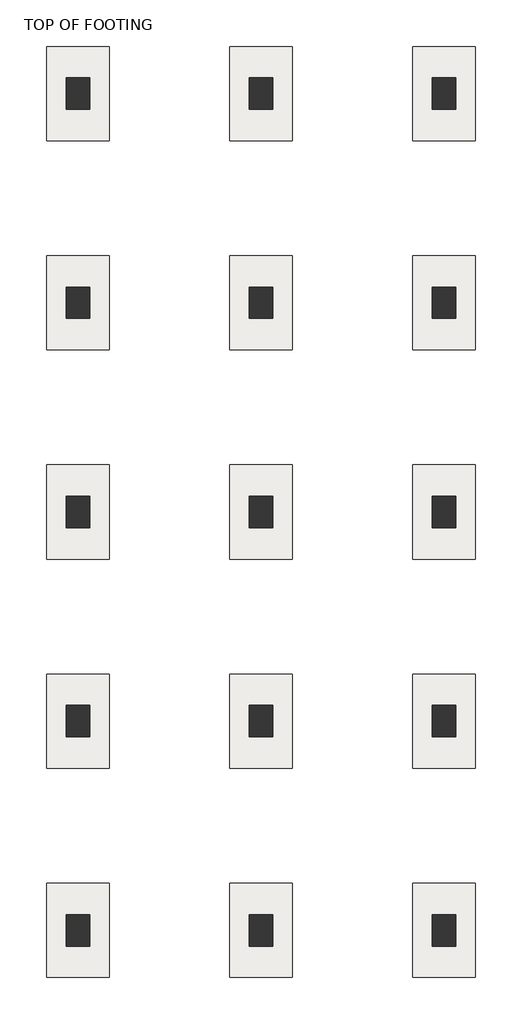
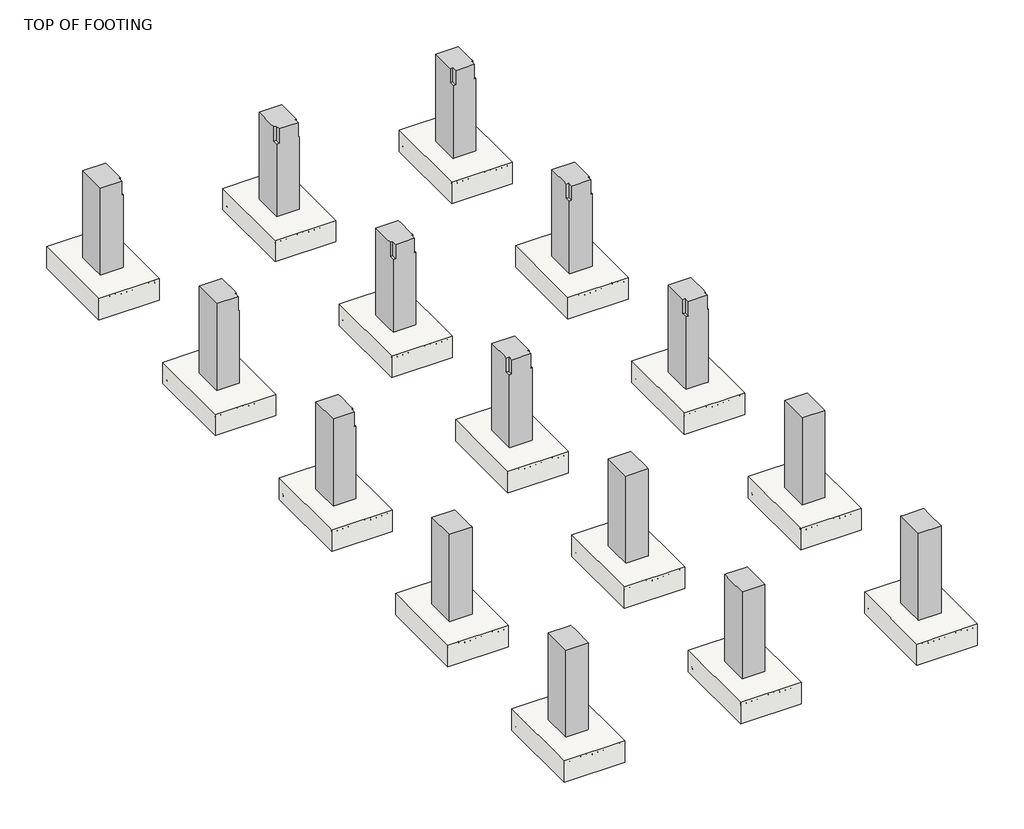
# One storey, part 1 of 11: 15 columns, 15 slabs.
"""IFC4 building model written with IfcOpenShell, lengths in millimetres."""

from ifc_helpers import new_model, si_unit, origin, place, context, project, spatial, faceted_brep, transform, mapped, element, save
from components import m_footing_rectangular_1800_x_1200_x_450mm_16ba7ea5

model = new_model("IFC4")

# Units and contexts
model_context = context("Model", 3, world=origin())
ifc_project = project(units=[si_unit("LENGTHUNIT", "METRE", prefix="MILLI")], contexts=[model_context])

# Site, building, storey
site = spatial("IfcSite", under=ifc_project)
building = spatial("IfcBuilding", under=site)
storey = spatial("IfcBuildingStorey", under=building, Name="TOP OF FOOTING", Elevation=-1828.8)

# Columns
placement = place(None, origin())
element("IfcColumn", 1, ObjectType="M_Concrete-Rectangular-Column : 450 x 600mm", at=placement, inside=storey, context=model_context, shape_type="Brep", body=[
    faceted_brep([(-9144.8884094, 19703.1212443, -1828.8), (-9144.8884094, 19103.1212443, -1828.8), (-9594.8884094, 19103.1212443, -1828.8), (-9594.8884094, 19703.1212443, -1828.8), (-9144.8884094, 19703.1212443, 0.0), (-9144.8884094, 19303.1212443, 0.0), (-9144.8884094, 19203.1212443, 0.0), (-9144.8884094, 19203.1212443, -300.0), (-9144.8884094, 19103.1212443, -300.0), (-9169.8884094, 19103.1212443, -300.0), (-9169.8884094, 19103.1212443, 0.0), (-9594.8884094, 19103.1212443, 0.0), (-9594.8884094, 19703.1212443, 0.0), (-9169.8884094, 19203.1212443, 0.0), (-9169.8884094, 19203.1212443, -300.0)], [[[0, 1, 2, 3]], [[1, 0, 4, 5, 6, 7, 8]], [[2, 1, 8, 9, 10, 11]], [[3, 2, 11, 12]], [[0, 3, 12, 4]], [[12, 11, 10, 13, 6, 5, 4]], [[7, 14, 9, 8]], [[14, 13, 10, 9]], [[14, 7, 6, 13]]]),
])
element("IfcColumn", 2, ObjectType="M_Concrete-Rectangular-Column : 450 x 600mm", at=placement, inside=storey, context=model_context, shape_type="Brep", body=[
    faceted_brep([(-5644.8884094, 19703.1212443, -1828.8), (-5644.8884094, 19103.1212443, -1828.8), (-6094.8884094, 19103.1212443, -1828.8), (-6094.8884094, 19703.1212443, -1828.8), (-5644.8884094, 19703.1212443, 0.0), (-5644.8884094, 19303.1212443, 0.0), (-5644.8884094, 19203.1212443, 0.0), (-5644.8884094, 19203.1212443, -300.0), (-5644.8884094, 19103.1212443, -300.0), (-5669.8884094, 19103.1212443, -300.0), (-5669.8884094, 19103.1212443, 0.0), (-6044.8884094, 19103.1212443, 0.0), (-6044.8884094, 19103.1212443, -300.0), (-6094.8884094, 19103.1212443, -300.0), (-6094.8884094, 19203.1212443, -300.0), (-6094.8884094, 19203.1212443, 0.0), (-6094.8884094, 19303.1212443, 0.0), (-6094.8884094, 19703.1212443, 0.0), (-6044.8884094, 19203.1212443, 0.0), (-5669.8884094, 19203.1212443, 0.0), (-5669.8884094, 19203.1212443, -300.0), (-6044.8884094, 19203.1212443, -300.0)], [[[0, 1, 2, 3]], [[1, 0, 4, 5, 6, 7, 8]], [[2, 1, 8, 9, 10, 11, 12, 13]], [[3, 2, 13, 14, 15, 16, 17]], [[0, 3, 17, 4]], [[4, 17, 16, 15, 18, 11, 10, 19, 6, 5]], [[7, 20, 9, 8]], [[20, 19, 10, 9]], [[20, 7, 6, 19]], [[21, 14, 13, 12]], [[18, 21, 12, 11]], [[14, 21, 18, 15]]]),
])
element("IfcColumn", 3, ObjectType="M_Concrete-Rectangular-Column : 450 x 600mm", at=placement, inside=storey, context=model_context, shape_type="Brep", body=[
    faceted_brep([(-2144.8884094, 19703.1212443, -1828.8), (-2144.8884094, 19103.1212443, -1828.8), (-2594.8884094, 19103.1212443, -1828.8), (-2594.8884094, 19703.1212443, -1828.8), (-2144.8884094, 19703.1212443, 0.0), (-2144.8884094, 19303.1212443, 0.0), (-2144.8884094, 19203.1212443, 0.0), (-2144.8884094, 19203.1212443, -300.0), (-2144.8884094, 19103.1212443, -300.0), (-2169.8884094, 19103.1212443, -300.0), (-2169.8884094, 19103.1212443, 0.0), (-2544.8884094, 19103.1212443, 0.0), (-2544.8884094, 19103.1212443, -300.0), (-2594.8884094, 19103.1212443, -300.0), (-2594.8884094, 19203.1212443, -300.0), (-2594.8884094, 19203.1212443, 0.0), (-2594.8884094, 19303.1212443, 0.0), (-2594.8884094, 19703.1212443, 0.0), (-2544.8884094, 19203.1212443, 0.0), (-2169.8884094, 19203.1212443, 0.0), (-2169.8884094, 19203.1212443, -300.0), (-2544.8884094, 19203.1212443, -300.0)], [[[0, 1, 2, 3]], [[1, 0, 4, 5, 6, 7, 8]], [[2, 1, 8, 9, 10, 11, 12, 13]], [[3, 2, 13, 14, 15, 16, 17]], [[0, 3, 17, 4]], [[4, 17, 16, 15, 18, 11, 10, 19, 6, 5]], [[7, 20, 9, 8]], [[20, 19, 10, 9]], [[20, 7, 6, 19]], [[21, 14, 13, 12]], [[18, 21, 12, 11]], [[14, 21, 18, 15]]]),
])
element("IfcColumn", 4, ObjectType="M_Concrete-Rectangular-Column : 450 x 600mm", at=placement, inside=storey, context=model_context, shape_type="Brep", body=[
    faceted_brep([(-9144.8884094, 15703.1212443, -1828.8), (-9144.8884094, 15103.1212443, -1828.8), (-9594.8884094, 15103.1212443, -1828.8), (-9594.8884094, 15703.1212443, -1828.8), (-9144.8884094, 15703.1212443, -300.0), (-9144.8884094, 15703.1212443, 0.0), (-9144.8884094, 15603.1212443, 0.0), (-9144.8884094, 15303.1212443, 0.0), (-9144.8884094, 15203.1212443, 0.0), (-9144.8884094, 15203.1212443, -300.0), (-9144.8884094, 15103.1212443, -300.0), (-9169.8884094, 15103.1212443, -300.0), (-9169.8884094, 15103.1212443, 0.0), (-9594.8884094, 15103.1212443, 0.0), (-9594.8884094, 15703.1212443, 0.0), (-9169.8884094, 15203.1212443, 0.0), (-9169.8884094, 15203.1212443, -300.0)], [[[0, 1, 2, 3]], [[1, 0, 4, 5, 6, 7, 8, 9, 10]], [[2, 1, 10, 11, 12, 13]], [[3, 2, 13, 14]], [[0, 3, 14, 5, 4]], [[14, 13, 12, 15, 8, 7, 6, 5]], [[9, 16, 11, 10]], [[16, 15, 12, 11]], [[16, 9, 8, 15]]]),
])
element("IfcColumn", 5, ObjectType="M_Concrete-Rectangular-Column : 450 x 600mm", at=placement, inside=storey, context=model_context, shape_type="Brep", body=[
    faceted_brep([(-5644.8884094, 15703.1212443, -1828.8), (-5644.8884094, 15103.1212443, -1828.8), (-6094.8884094, 15103.1212443, -1828.8), (-6094.8884094, 15703.1212443, -1828.8), (-5644.8884094, 15703.1212443, -300.0), (-5644.8884094, 15703.1212443, 0.0), (-5644.8884094, 15603.1212443, 0.0), (-5644.8884094, 15303.1212443, 0.0), (-5644.8884094, 15203.1212443, 0.0), (-5644.8884094, 15203.1212443, -300.0), (-5644.8884094, 15103.1212443, -300.0), (-5669.8884094, 15103.1212443, -300.0), (-5669.8884094, 15103.1212443, 0.0), (-6044.8884094, 15103.1212443, 0.0), (-6044.8884094, 15103.1212443, -300.0), (-6094.8884094, 15103.1212443, -300.0), (-6094.8884094, 15203.1212443, -300.0), (-6094.8884094, 15203.1212443, 0.0), (-6094.8884094, 15303.1212443, 0.0), (-6094.8884094, 15603.1212443, 0.0), (-6094.8884094, 15703.1212443, 0.0), (-6094.8884094, 15703.1212443, -300.0), (-6044.8884094, 15203.1212443, 0.0), (-5669.8884094, 15203.1212443, 0.0), (-6044.8884094, 15203.1212443, -300.0), (-5669.8884094, 15203.1212443, -300.0)], [[[0, 1, 2, 3]], [[1, 0, 4, 5, 6, 7, 8, 9, 10]], [[2, 1, 10, 11, 12, 13, 14, 15]], [[3, 2, 15, 16, 17, 18, 19, 20, 21]], [[0, 3, 21, 20, 5, 4]], [[5, 20, 19, 18, 17, 22, 13, 12, 23, 8, 7, 6]], [[24, 16, 15, 14]], [[22, 24, 14, 13]], [[16, 24, 22, 17]], [[9, 25, 11, 10]], [[25, 23, 12, 11]], [[25, 9, 8, 23]]]),
])
element("IfcColumn", 6, ObjectType="M_Concrete-Rectangular-Column : 450 x 600mm", at=placement, inside=storey, context=model_context, shape_type="Brep", body=[
    faceted_brep([(-2144.8884094, 15703.1212443, -1828.8), (-2144.8884094, 15103.1212443, -1828.8), (-2594.8884094, 15103.1212443, -1828.8), (-2594.8884094, 15703.1212443, -1828.8), (-2144.8884094, 15703.1212443, -300.0), (-2144.8884094, 15703.1212443, 0.0), (-2144.8884094, 15603.1212443, 0.0), (-2144.8884094, 15303.1212443, 0.0), (-2144.8884094, 15203.1212443, 0.0), (-2144.8884094, 15203.1212443, -300.0), (-2144.8884094, 15103.1212443, -300.0), (-2169.8884094, 15103.1212443, -300.0), (-2169.8884094, 15103.1212443, 0.0), (-2544.8884094, 15103.1212443, 0.0), (-2544.8884094, 15103.1212443, -300.0), (-2594.8884094, 15103.1212443, -300.0), (-2594.8884094, 15203.1212443, -300.0), (-2594.8884094, 15203.1212443, 0.0), (-2594.8884094, 15303.1212443, 0.0), (-2594.8884094, 15603.1212443, 0.0), (-2594.8884094, 15703.1212443, 0.0), (-2594.8884094, 15703.1212443, -300.0), (-2544.8884094, 15203.1212443, 0.0), (-2169.8884094, 15203.1212443, 0.0), (-2169.8884094, 15203.1212443, -300.0), (-2544.8884094, 15203.1212443, -300.0)], [[[0, 1, 2, 3]], [[1, 0, 4, 5, 6, 7, 8, 9, 10]], [[2, 1, 10, 11, 12, 13, 14, 15]], [[3, 2, 15, 16, 17, 18, 19, 20, 21]], [[0, 3, 21, 20, 5, 4]], [[5, 20, 19, 18, 17, 22, 13, 12, 23, 8, 7, 6]], [[9, 24, 11, 10]], [[24, 23, 12, 11]], [[24, 9, 8, 23]], [[25, 16, 15, 14]], [[22, 25, 14, 13]], [[16, 25, 22, 17]]]),
])
element("IfcColumn", 7, ObjectType="M_Concrete-Rectangular-Column : 450 x 600mm", at=placement, inside=storey, context=model_context, shape_type="Brep", body=[
    faceted_brep([(-9144.8884094, 11703.1212443, -1828.8), (-9144.8884094, 11103.1212443, -1828.8), (-9594.8884094, 11103.1212443, -1828.8), (-9594.8884094, 11703.1212443, -1828.8), (-9144.8884094, 11703.1212443, -300.0), (-9144.8884094, 11703.1212443, 0.0), (-9144.8884094, 11603.1212443, 0.0), (-9144.8884094, 11303.1212443, 0.0), (-9144.8884094, 11203.1212443, 0.0), (-9144.8884094, 11203.1212443, -300.0), (-9144.8884094, 11103.1212443, -300.0), (-9169.8884094, 11103.1212443, -300.0), (-9169.8884094, 11103.1212443, 0.0), (-9594.8884094, 11103.1212443, 0.0), (-9594.8884094, 11703.1212443, 0.0), (-9169.8884094, 11203.1212443, 0.0), (-9169.8884094, 11203.1212443, -300.0)], [[[0, 1, 2, 3]], [[1, 0, 4, 5, 6, 7, 8, 9, 10]], [[2, 1, 10, 11, 12, 13]], [[3, 2, 13, 14]], [[0, 3, 14, 5, 4]], [[14, 13, 12, 15, 8, 7, 6, 5]], [[9, 16, 11, 10]], [[16, 15, 12, 11]], [[16, 9, 8, 15]]]),
])
element("IfcColumn", 8, ObjectType="M_Concrete-Rectangular-Column : 450 x 600mm", at=placement, inside=storey, context=model_context, shape_type="Brep", body=[
    faceted_brep([(-5644.8884094, 11703.1212443, -1828.8), (-5644.8884094, 11103.1212443, -1828.8), (-6094.8884094, 11103.1212443, -1828.8), (-6094.8884094, 11703.1212443, -1828.8), (-5644.8884094, 11703.1212443, -300.0), (-5644.8884094, 11703.1212443, 0.0), (-5644.8884094, 11603.1212443, 0.0), (-5644.8884094, 11303.1212443, 0.0), (-5644.8884094, 11203.1212443, 0.0), (-5644.8884094, 11203.1212443, -300.0), (-5644.8884094, 11103.1212443, -300.0), (-5669.8884094, 11103.1212443, -300.0), (-5669.8884094, 11103.1212443, 0.0), (-6044.8884094, 11103.1212443, 0.0), (-6044.8884094, 11103.1212443, -300.0), (-6094.8884094, 11103.1212443, -300.0), (-6094.8884094, 11203.1212443, -300.0), (-6094.8884094, 11203.1212443, 0.0), (-6094.8884094, 11303.1212443, 0.0), (-6094.8884094, 11603.1212443, 0.0), (-6094.8884094, 11703.1212443, 0.0), (-6094.8884094, 11703.1212443, -300.0), (-6044.8884094, 11203.1212443, 0.0), (-5669.8884094, 11203.1212443, 0.0), (-5669.8884094, 11203.1212443, -300.0), (-6044.8884094, 11203.1212443, -300.0)], [[[0, 1, 2, 3]], [[1, 0, 4, 5, 6, 7, 8, 9, 10]], [[2, 1, 10, 11, 12, 13, 14, 15]], [[3, 2, 15, 16, 17, 18, 19, 20, 21]], [[0, 3, 21, 20, 5, 4]], [[5, 20, 19, 18, 17, 22, 13, 12, 23, 8, 7, 6]], [[9, 24, 11, 10]], [[24, 23, 12, 11]], [[24, 9, 8, 23]], [[25, 16, 15, 14]], [[22, 25, 14, 13]], [[16, 25, 22, 17]]]),
])
element("IfcColumn", 9, ObjectType="M_Concrete-Rectangular-Column : 450 x 600mm", at=placement, inside=storey, context=model_context, shape_type="Brep", body=[
    faceted_brep([(-2144.8884094, 11703.1212443, -1828.8), (-2144.8884094, 11103.1212443, -1828.8), (-2594.8884094, 11103.1212443, -1828.8), (-2594.8884094, 11703.1212443, -1828.8), (-2144.8884094, 11703.1212443, -300.0), (-2144.8884094, 11703.1212443, 0.0), (-2144.8884094, 11603.1212443, 0.0), (-2144.8884094, 11303.1212443, 0.0), (-2144.8884094, 11203.1212443, 0.0), (-2144.8884094, 11203.1212443, -300.0), (-2144.8884094, 11103.1212443, -300.0), (-2169.8884094, 11103.1212443, -300.0), (-2169.8884094, 11103.1212443, 0.0), (-2544.8884094, 11103.1212443, 0.0), (-2544.8884094, 11103.1212443, -300.0), (-2594.8884094, 11103.1212443, -300.0), (-2594.8884094, 11203.1212443, -300.0), (-2594.8884094, 11203.1212443, 0.0), (-2594.8884094, 11303.1212443, 0.0), (-2594.8884094, 11603.1212443, 0.0), (-2594.8884094, 11703.1212443, 0.0), (-2594.8884094, 11703.1212443, -300.0), (-2544.8884094, 11203.1212443, 0.0), (-2169.8884094, 11203.1212443, 0.0), (-2169.8884094, 11203.1212443, -300.0), (-2544.8884094, 11203.1212443, -300.0)], [[[0, 1, 2, 3]], [[1, 0, 4, 5, 6, 7, 8, 9, 10]], [[2, 1, 10, 11, 12, 13, 14, 15]], [[3, 2, 15, 16, 17, 18, 19, 20, 21]], [[0, 3, 21, 20, 5, 4]], [[5, 20, 19, 18, 17, 22, 13, 12, 23, 8, 7, 6]], [[9, 24, 11, 10]], [[24, 23, 12, 11]], [[24, 9, 8, 23]], [[25, 16, 15, 14]], [[22, 25, 14, 13]], [[16, 25, 22, 17]]]),
])
element("IfcColumn", 10, ObjectType="M_Concrete-Rectangular-Column : 450 x 600mm", at=placement, inside=storey, context=model_context, shape_type="Brep", body=[
    faceted_brep([(-9144.8884094, 7703.1212443, -1828.8), (-9144.8884094, 7103.1212443, -1828.8), (-9594.8884094, 7103.1212443, -1828.8), (-9594.8884094, 7703.1212443, -1828.8), (-9144.8884094, 7703.1212443, -300.0), (-9144.8884094, 7703.1212443, 0.0), (-9144.8884094, 7603.1212443, 0.0), (-9144.8884094, 7203.1212443, 0.0), (-9144.8884094, 7103.1212443, 0.0), (-9144.8884094, 7103.1212443, -300.0), (-9169.8884094, 7103.1212443, 0.0), (-9594.8884094, 7103.1212443, 0.0), (-9594.8884094, 7703.1212443, 0.0)], [[[0, 1, 2, 3]], [[1, 0, 4, 5, 6, 7, 8, 9]], [[2, 1, 9, 8, 10, 11]], [[3, 2, 11, 12]], [[0, 3, 12, 5, 4]], [[12, 11, 10, 8, 7, 6, 5]]]),
])
element("IfcColumn", 11, ObjectType="M_Concrete-Rectangular-Column : 450 x 600mm", at=placement, inside=storey, context=model_context, shape_type="Brep", body=[
    faceted_brep([(-5644.8884094, 7703.1212443, -1828.8), (-5644.8884094, 7103.1212443, -1828.8), (-6094.8884094, 7103.1212443, -1828.8), (-6094.8884094, 7703.1212443, -1828.8), (-5644.8884094, 7703.1212443, -300.0), (-5644.8884094, 7703.1212443, 0.0), (-5644.8884094, 7603.1212443, 0.0), (-5644.8884094, 7203.1212443, 0.0), (-5644.8884094, 7103.1212443, 0.0), (-5644.8884094, 7103.1212443, -300.0), (-5669.8884094, 7103.1212443, 0.0), (-6044.8884094, 7103.1212443, 0.0), (-6094.8884094, 7103.1212443, 0.0), (-6094.8884094, 7103.1212443, -300.0), (-6094.8884094, 7203.1212443, 0.0), (-6094.8884094, 7603.1212443, 0.0), (-6094.8884094, 7703.1212443, 0.0), (-6094.8884094, 7703.1212443, -300.0)], [[[0, 1, 2, 3]], [[1, 0, 4, 5, 6, 7, 8, 9]], [[2, 1, 9, 8, 10, 11, 12, 13]], [[3, 2, 13, 12, 14, 15, 16, 17]], [[0, 3, 17, 16, 5, 4]], [[5, 16, 15, 14, 12, 11, 10, 8, 7, 6]]]),
])
element("IfcColumn", 12, ObjectType="M_Concrete-Rectangular-Column : 450 x 600mm", at=placement, inside=storey, context=model_context, shape_type="Brep", body=[
    faceted_brep([(-2144.8884094, 7703.1212443, -1828.8), (-2144.8884094, 7103.1212443, -1828.8), (-2594.8884094, 7103.1212443, -1828.8), (-2594.8884094, 7703.1212443, -1828.8), (-2144.8884094, 7703.1212443, -300.0), (-2144.8884094, 7703.1212443, 0.0), (-2144.8884094, 7603.1212443, 0.0), (-2144.8884094, 7203.1212443, 0.0), (-2144.8884094, 7103.1212443, 0.0), (-2144.8884094, 7103.1212443, -300.0), (-2169.8884094, 7103.1212443, 0.0), (-2544.8884094, 7103.1212443, 0.0), (-2594.8884094, 7103.1212443, 0.0), (-2594.8884094, 7103.1212443, -300.0), (-2594.8884094, 7203.1212443, 0.0), (-2594.8884094, 7603.1212443, 0.0), (-2594.8884094, 7703.1212443, 0.0), (-2594.8884094, 7703.1212443, -300.0)], [[[0, 1, 2, 3]], [[1, 0, 4, 5, 6, 7, 8, 9]], [[2, 1, 9, 8, 10, 11, 12, 13]], [[3, 2, 13, 12, 14, 15, 16, 17]], [[0, 3, 17, 16, 5, 4]], [[5, 16, 15, 14, 12, 11, 10, 8, 7, 6]]]),
])
element("IfcColumn", 13, ObjectType="M_Concrete-Rectangular-Column : 450 x 600mm", at=placement, inside=storey, context=model_context, shape_type="Brep", body=[
    faceted_brep([(-9144.8884094, 3703.1212443, -1828.8), (-9144.8884094, 3103.1212443, -1828.8), (-9594.8884094, 3103.1212443, -1828.8), (-9594.8884094, 3703.1212443, -1828.8), (-9144.8884094, 3703.1212443, -300.0), (-9144.8884094, 3703.1212443, 0.0), (-9144.8884094, 3503.1212443, 0.0), (-9144.8884094, 3103.1212443, 0.0), (-9594.8884094, 3103.1212443, 0.0), (-9594.8884094, 3703.1212443, 0.0), (-9169.8884094, 3703.1212443, 0.0)], [[[0, 1, 2, 3]], [[1, 0, 4, 5, 6, 7]], [[2, 1, 7, 8]], [[3, 2, 8, 9]], [[0, 3, 9, 10, 5, 4]], [[8, 7, 6, 5, 10, 9]]]),
])
element("IfcColumn", 14, ObjectType="M_Concrete-Rectangular-Column : 450 x 600mm", at=placement, inside=storey, context=model_context, shape_type="Brep", body=[
    faceted_brep([(-5644.8884094, 3703.1212443, -1828.8), (-5644.8884094, 3103.1212443, -1828.8), (-6094.8884094, 3103.1212443, -1828.8), (-6094.8884094, 3703.1212443, -1828.8), (-5644.8884094, 3703.1212443, -300.0), (-5644.8884094, 3703.1212443, 0.0), (-5644.8884094, 3503.1212443, 0.0), (-5644.8884094, 3103.1212443, 0.0), (-6094.8884094, 3103.1212443, 0.0), (-6094.8884094, 3503.1212443, 0.0), (-6094.8884094, 3703.1212443, 0.0), (-6094.8884094, 3703.1212443, -300.0), (-6044.8884094, 3703.1212443, 0.0), (-5669.8884094, 3703.1212443, 0.0)], [[[0, 1, 2, 3]], [[1, 0, 4, 5, 6, 7]], [[2, 1, 7, 8]], [[3, 2, 8, 9, 10, 11]], [[0, 3, 11, 10, 12, 13, 5, 4]], [[8, 7, 6, 5, 13, 12, 10, 9]]]),
])
element("IfcColumn", 15, ObjectType="M_Concrete-Rectangular-Column : 450 x 600mm", at=placement, inside=storey, context=model_context, shape_type="Brep", body=[
    faceted_brep([(-2144.8884094, 3703.1212443, -1828.8), (-2144.8884094, 3103.1212443, -1828.8), (-2594.8884094, 3103.1212443, -1828.8), (-2594.8884094, 3703.1212443, -1828.8), (-2144.8884094, 3703.1212443, -300.0), (-2144.8884094, 3703.1212443, 0.0), (-2144.8884094, 3503.1212443, 0.0), (-2144.8884094, 3103.1212443, 0.0), (-2594.8884094, 3103.1212443, 0.0), (-2594.8884094, 3503.1212443, 0.0), (-2594.8884094, 3703.1212443, 0.0), (-2594.8884094, 3703.1212443, -300.0), (-2544.8884094, 3703.1212443, 0.0), (-2169.8884094, 3703.1212443, 0.0)], [[[0, 1, 2, 3]], [[1, 0, 4, 5, 6, 7]], [[2, 1, 7, 8]], [[3, 2, 8, 9, 10, 11]], [[0, 3, 11, 10, 12, 13, 5, 4]], [[8, 7, 6, 5, 13, 12, 10, 9]]]),
])

# Slabs
m_footing_rectangular_1800_x_1200_x_450mm_shape = m_footing_rectangular_1800_x_1200_x_450mm_16ba7ea5(model_context)
element("IfcSlab", 16, ObjectType="M_Footing-Rectangular : 1800 x 1200 x 450mm", at=placement, inside=storey, context=model_context, shape_type="MappedRepresentation", body=[
    mapped(m_footing_rectangular_1800_x_1200_x_450mm_shape, transform((-9369.8884094, 19403.1212443, -1828.8), x_axis=(1.0, 0.0, 0.0), y_axis=(0.0, 1.0, 0.0), z_axis=(0.0, 0.0, 1.0))),
])
element("IfcSlab", 17, ObjectType="M_Footing-Rectangular : 1800 x 1200 x 450mm", at=placement, inside=storey, context=model_context, shape_type="MappedRepresentation", body=[
    mapped(m_footing_rectangular_1800_x_1200_x_450mm_shape, transform((-5869.8884094, 19403.1212443, -1828.8), x_axis=(1.0, 0.0, 0.0), y_axis=(0.0, 1.0, 0.0), z_axis=(0.0, 0.0, 1.0))),
])
element("IfcSlab", 18, ObjectType="M_Footing-Rectangular : 1800 x 1200 x 450mm", at=placement, inside=storey, context=model_context, shape_type="MappedRepresentation", body=[
    mapped(m_footing_rectangular_1800_x_1200_x_450mm_shape, transform((-2369.8884094, 19403.1212443, -1828.8), x_axis=(1.0, 0.0, 0.0), y_axis=(0.0, 1.0, 0.0), z_axis=(0.0, 0.0, 1.0))),
])
element("IfcSlab", 19, ObjectType="M_Footing-Rectangular : 1800 x 1200 x 450mm", at=placement, inside=storey, context=model_context, shape_type="MappedRepresentation", body=[
    mapped(m_footing_rectangular_1800_x_1200_x_450mm_shape, transform((-9369.8884094, 3403.1212443, -1828.8), x_axis=(1.0, 0.0, 0.0), y_axis=(0.0, 1.0, 0.0), z_axis=(0.0, 0.0, 1.0))),
])
element("IfcSlab", 20, ObjectType="M_Footing-Rectangular : 1800 x 1200 x 450mm", at=placement, inside=storey, context=model_context, shape_type="MappedRepresentation", body=[
    mapped(m_footing_rectangular_1800_x_1200_x_450mm_shape, transform((-5869.8884094, 3403.1212443, -1828.8), x_axis=(1.0, 0.0, 0.0), y_axis=(0.0, 1.0, 0.0), z_axis=(0.0, 0.0, 1.0))),
])
element("IfcSlab", 21, ObjectType="M_Footing-Rectangular : 1800 x 1200 x 450mm", at=placement, inside=storey, context=model_context, shape_type="MappedRepresentation", body=[
    mapped(m_footing_rectangular_1800_x_1200_x_450mm_shape, transform((-2369.8884094, 3403.1212443, -1828.8), x_axis=(1.0, 0.0, 0.0), y_axis=(0.0, 1.0, 0.0), z_axis=(0.0, 0.0, 1.0))),
])
element("IfcSlab", 22, ObjectType="M_Footing-Rectangular : 1800 x 1200 x 450mm", at=placement, inside=storey, context=model_context, shape_type="MappedRepresentation", body=[
    mapped(m_footing_rectangular_1800_x_1200_x_450mm_shape, transform((-2369.8884094, 7403.1212443, -1828.8), x_axis=(1.0, 0.0, 0.0), y_axis=(0.0, 1.0, 0.0), z_axis=(0.0, 0.0, 1.0))),
])
element("IfcSlab", 23, ObjectType="M_Footing-Rectangular : 1800 x 1200 x 450mm", at=placement, inside=storey, context=model_context, shape_type="MappedRepresentation", body=[
    mapped(m_footing_rectangular_1800_x_1200_x_450mm_shape, transform((-5869.8884094, 7403.1212443, -1828.8), x_axis=(1.0, 0.0, 0.0), y_axis=(0.0, 1.0, 0.0), z_axis=(0.0, 0.0, 1.0))),
])
element("IfcSlab", 24, ObjectType="M_Footing-Rectangular : 1800 x 1200 x 450mm", at=placement, inside=storey, context=model_context, shape_type="MappedRepresentation", body=[
    mapped(m_footing_rectangular_1800_x_1200_x_450mm_shape, transform((-9369.8884094, 7403.1212443, -1828.8), x_axis=(1.0, 0.0, 0.0), y_axis=(0.0, 1.0, 0.0), z_axis=(0.0, 0.0, 1.0))),
])
element("IfcSlab", 25, ObjectType="M_Footing-Rectangular : 1800 x 1200 x 450mm", at=placement, inside=storey, context=model_context, shape_type="MappedRepresentation", body=[
    mapped(m_footing_rectangular_1800_x_1200_x_450mm_shape, transform((-9369.8884094, 11403.1212443, -1828.8), x_axis=(1.0, 0.0, 0.0), y_axis=(0.0, 1.0, 0.0), z_axis=(0.0, 0.0, 1.0))),
])
element("IfcSlab", 26, ObjectType="M_Footing-Rectangular : 1800 x 1200 x 450mm", at=placement, inside=storey, context=model_context, shape_type="MappedRepresentation", body=[
    mapped(m_footing_rectangular_1800_x_1200_x_450mm_shape, transform((-5869.8884094, 11403.1212443, -1828.8), x_axis=(1.0, 0.0, 0.0), y_axis=(0.0, 1.0, 0.0), z_axis=(0.0, 0.0, 1.0))),
])
element("IfcSlab", 27, ObjectType="M_Footing-Rectangular : 1800 x 1200 x 450mm", at=placement, inside=storey, context=model_context, shape_type="MappedRepresentation", body=[
    mapped(m_footing_rectangular_1800_x_1200_x_450mm_shape, transform((-2369.8884094, 11403.1212443, -1828.8), x_axis=(1.0, 0.0, 0.0), y_axis=(0.0, 1.0, 0.0), z_axis=(0.0, 0.0, 1.0))),
])
element("IfcSlab", 28, ObjectType="M_Footing-Rectangular : 1800 x 1200 x 450mm", at=placement, inside=storey, context=model_context, shape_type="MappedRepresentation", body=[
    mapped(m_footing_rectangular_1800_x_1200_x_450mm_shape, transform((-2369.8884094, 15403.1212443, -1828.8), x_axis=(1.0, 0.0, 0.0), y_axis=(0.0, 1.0, 0.0), z_axis=(0.0, 0.0, 1.0))),
])
element("IfcSlab", 29, ObjectType="M_Footing-Rectangular : 1800 x 1200 x 450mm", at=placement, inside=storey, context=model_context, shape_type="MappedRepresentation", body=[
    mapped(m_footing_rectangular_1800_x_1200_x_450mm_shape, transform((-5869.8884094, 15403.1212443, -1828.8), x_axis=(1.0, 0.0, 0.0), y_axis=(0.0, 1.0, 0.0), z_axis=(0.0, 0.0, 1.0))),
])
element("IfcSlab", 30, ObjectType="M_Footing-Rectangular : 1800 x 1200 x 450mm", at=placement, inside=storey, context=model_context, shape_type="MappedRepresentation", body=[
    mapped(m_footing_rectangular_1800_x_1200_x_450mm_shape, transform((-9369.8884094, 15403.1212443, -1828.8), x_axis=(1.0, 0.0, 0.0), y_axis=(0.0, 1.0, 0.0), z_axis=(0.0, 0.0, 1.0))),
])

save(model, "model.ifc")

# Revit data of these elements
# Grids (mm)
#   "1": line (-9369.888, 27561.518) -> (-9369.888, -7707.002)
#   "2": line (-5869.888, 27561.518) -> (-5869.888, -7707.002)
#   "3": line (-2369.888, 27561.518) -> (-2369.888, -7707.002)
#   "4": line (1130.112, 27561.518) -> (1130.112, -7707.002)
#   "5": line (4630.112, 27561.518) -> (4630.112, -7707.002)
#   "6": line (8130.112, 27561.518) -> (8130.112, -7707.002)
#   "A": line (24627.262, 19403.121) -> (-10860.54, 19403.121)
#   "B": line (24627.262, 15403.121) -> (-10860.54, 15403.121)
#   "C": line (24627.262, 11403.121) -> (-10860.54, 11403.121)
#   "D": line (24627.262, 7403.121) -> (-10860.54, 7403.121)
#   "E": line (24627.262, 3403.121) -> (-10860.54, 3403.121)
# Type "M_Concrete-Rectangular-Column : 450 x 600mm"
#   b = 1' - 5.71654"
#   h = 1' - 11.62205"
#   Structural Material [instance default] = Concrete, Cast-in-Place gray
# Type "M_Footing-Rectangular : 1800 x 1200 x 450mm"
#   Width = 3' - 11.24409"
#   Length = 5' - 10.86614"
#   Foundation Thickness = 1' - 5.71654"
#   Structural Material [instance default] = Concrete, Cast-in-Place gray
#   Assembly Code = ""
# Elements 1, 2, 3, 4, 5, 6, 7, 8, 9, 10, 11, 12, 13, 14, 15 (IfcColumn, "M_Concrete-Rectangular-Column : 450 x 600mm")
#   Structural Material = Concrete, Cast-in-Place gray
#   Phase Created = New Construction
#   Materials on its faces: "Concrete, Cast-in-Place gray"
# Elements 16, 17, 18, 19, 20, 21, 22, 23, 24, 25, 26, 27, 28, 29, 30 (IfcSlab, "M_Footing-Rectangular : 1800 x 1200 x 450mm")
#   Structural Material = Concrete, Cast-in-Place gray
#   Phase Created = New Construction
#   Materials on its faces: "Concrete, Cast-in-Place gray"
# Materials
#   "Concrete, Cast-in-Place gray": class "Concrete", colour RGB 192 192 192, transparency 0, Description = "Cast-in-place concrete", Cost = 0
